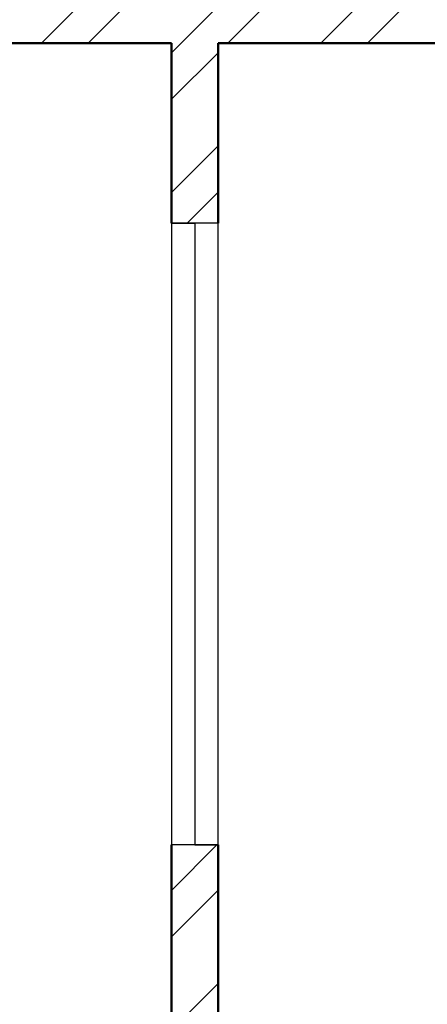
# Model space of a CAD drawing. Units: inches. Extents: x 963 to 2075, y 289 to 2657.
# Tile 61 of 98: x 1149 to 1188, y 2230 to 2325. Entities that reach past the tile are written whole.
import ezdxf

# ---------------------------------------------------------------- set-up
doc = ezdxf.new("R2010")
doc.units = ezdxf.units.IN
for name, color, linetype, lineweight in [('A-GLAZ', 3, 'Continuous', 25), ('A-WALL', 7, 'Continuous', 50), ('A-WALL-PATT', 8, 'Continuous', 13)]:
    doc.layers.add(name, color=color, linetype=linetype, lineweight=lineweight)

msp = doc.modelspace()

# ---------------------------------------------------------------- hatches: boundary and pattern name
at = {"layer": 'A-WALL-PATT'}
h = msp.add_hatch(dxfattribs=at)
h.set_pattern_fill('ANSI32', color=256)
h.paths.add_polyline_path([(1296.922, 2558.318), (1203.922, 2558.318), (1203.922, 2493.818), (1191.533, 2493.818), (1191.533, 2489.318), (1211.063, 2489.318), (1211.063, 2492.02), (1211.063, 2493.818), (1208.422, 2493.818), (1208.422, 2553.818), (1292.422, 2553.818), (1292.422, 2538.863), (1296.922, 2538.863)])
h.paths.add_polyline_path([(1442.422, 2558.318), (1349.422, 2558.318), (1349.422, 2538.943), (1353.922, 2538.943), (1353.922, 2553.818), (1437.922, 2553.818), (1437.922, 2493.818), (1434.542, 2493.818), (1434.542, 2489.318), (1448.311, 2489.318), (1448.311, 2491.568), (1448.311, 2493.818), (1442.422, 2493.818)])
h.paths.add_polyline_path([(1415.554, 2491.568), (1415.554, 2493.818), (1340.941, 2493.818), (1340.941, 2489.318), (1371.922, 2489.318), (1371.922, 2378.318), (1367.596, 2378.318), (1367.596, 2373.818), (1371.922, 2373.818), (1371.922, 2355.185), (1376.422, 2355.185), (1376.422, 2489.318), (1415.554, 2489.318)])
h.paths.add_polyline_path([(1304.941, 2491.568), (1304.941, 2493.818), (1296.922, 2493.818), (1296.922, 2514.863), (1292.422, 2514.863), (1292.422, 2493.818), (1232.808, 2493.818), (1232.808, 2489.318), (1256.422, 2489.318), (1256.422, 2327.318), (1253.714, 2327.318), (1253.714, 2322.818), (1328.422, 2322.818), (1328.422, 2331.147), (1323.922, 2331.147), (1323.922, 2327.318), (1260.922, 2327.318), (1260.922, 2373.818), (1323.922, 2373.818), (1323.922, 2357.812), (1328.422, 2357.812), (1328.422, 2373.818), (1346.007, 2373.818), (1346.007, 2376.068), (1346.007, 2378.318), (1260.922, 2378.318), (1260.922, 2489.318), (1304.941, 2489.318)])
h.paths.add_polyline_path([(1226.654, 2327.318), (1124.422, 2327.318), (1124.422, 2347.447), (1119.922, 2347.447), (1119.922, 2322.818), (1163.422, 2322.818), (1163.422, 2305.435), (1165.672, 2305.435), (1167.922, 2305.435), (1167.922, 2322.818), (1226.654, 2322.818), (1226.654, 2325.068)])
h.paths.add_polyline_path([(1095.922, 2489.318), (1124.422, 2489.318), (1131.533, 2489.318), (1131.533, 2491.568), (1131.533, 2493.818), (1119.922, 2493.818), (1091.422, 2493.818), (1091.422, 2417.318), (1095.922, 2417.318), (1119.922, 2417.318), (1119.922, 2407.447), (1124.422, 2407.447), (1124.422, 2421.818), (1095.922, 2421.818)])
h.paths.add_polyline_path([(1512.922, 2558.318), (1508.422, 2558.318), (1508.422, 2493.818), (1503.401, 2493.818), (1503.401, 2489.318), (1508.422, 2489.318), (1508.422, 2327.318), (1376.422, 2327.318), (1376.422, 2330.273), (1371.922, 2330.273), (1371.922, 2298.744), (1376.422, 2298.744), (1376.422, 2322.818), (1508.422, 2322.818), (1508.422, 2165.318), (1504.255, 2165.318), (1504.255, 2160.818), (1508.422, 2160.818), (1508.422, 2108.318), (1512.922, 2108.318), (1512.922, 2160.818), (1516.182, 2160.818), (1516.182, 2163.068), (1516.182, 2165.318), (1512.922, 2165.318), (1512.922, 2322.818), (1644.922, 2322.818), (1644.922, 2298.744), (1649.422, 2298.744), (1649.422, 2322.818), (1649.422, 2330.944), (1647.172, 2330.944), (1644.922, 2330.944), (1644.922, 2327.318), (1512.922, 2327.318), (1512.922, 2489.318), (1516.759, 2489.318), (1516.759, 2491.568), (1516.759, 2493.818), (1512.922, 2493.818)])
h.paths.add_polyline_path([(1671.922, 2558.318), (1578.922, 2558.318), (1578.922, 2493.818), (1573.526, 2493.818), (1573.526, 2489.318), (1586.537, 2489.318), (1586.537, 2491.568), (1586.537, 2493.818), (1583.422, 2493.818), (1583.422, 2553.818), (1667.422, 2553.818), (1667.422, 2541.109), (1671.922, 2541.109)])
h.paths.add_polyline_path([(1681.257, 2493.818), (1671.922, 2493.818), (1671.922, 2517.109), (1667.422, 2517.109), (1667.422, 2493.818), (1610.218, 2493.818), (1610.218, 2489.318), (1644.922, 2489.318), (1644.922, 2357.865), (1649.422, 2357.865), (1649.422, 2373.818), (1652.203, 2373.818), (1652.203, 2375.827), (1652.203, 2378.318), (1649.422, 2378.318), (1649.422, 2489.318), (1681.257, 2489.318), (1681.257, 2491.568)])
h.paths.add_polyline_path([(1821.922, 2558.318), (1728.922, 2558.318), (1728.922, 2541), (1733.422, 2541), (1733.422, 2553.818), (1817.422, 2553.818), (1817.422, 2493.818), (1813.507, 2493.818), (1813.507, 2489.318), (1830.078, 2489.318), (1830.078, 2491.568), (1830.078, 2493.818), (1821.922, 2493.818)])
h.paths.add_polyline_path([(1794.244, 2493.818), (1717.257, 2493.818), (1717.257, 2489.318), (1760.422, 2489.318), (1760.422, 2378.318), (1674.401, 2378.318), (1674.401, 2373.818), (1692.922, 2373.818), (1692.922, 2356.954), (1697.422, 2356.954), (1697.422, 2373.818), (1760.422, 2373.818), (1760.422, 2327.318), (1697.422, 2327.318), (1697.422, 2333.341), (1692.922, 2333.341), (1692.922, 2322.818), (1768.037, 2322.818), (1768.037, 2325.068), (1768.037, 2327.318), (1764.922, 2327.318), (1764.922, 2489.318), (1794.244, 2489.318)])
h.paths.add_polyline_path([(1733.422, 2517), (1728.922, 2517), (1728.922, 2493.818), (1733.422, 2493.818)], flags=17)
h.paths.add_polyline_path([(1929.922, 2493.818), (1890.078, 2493.818), (1890.078, 2489.318), (1896.922, 2489.318), (1925.422, 2489.318), (1925.422, 2421.818), (1896.922, 2421.818), (1896.922, 2408.318), (1901.422, 2408.318), (1901.422, 2417.318), (1925.422, 2417.318), (1929.922, 2417.318)])
h.paths.add_polyline_path([(1901.422, 2348.318), (1896.922, 2348.318), (1896.922, 2327.318), (1800.423, 2327.318), (1800.423, 2322.818), (1853.422, 2322.818), (1853.422, 2309.453), (1857.922, 2309.453), (1857.922, 2322.818), (1901.422, 2322.818)])
h.paths.add_polyline_path([(1857.922, 2249.453), (1853.422, 2249.453), (1853.422, 2214.818), (1686.309, 2214.818), (1686.309, 2210.318), (1853.422, 2210.318), (1853.422, 2202.134), (1857.922, 2202.134), (1857.922, 2210.318)])
h.paths.add_polyline_path([(1857.922, 2142.134), (1853.422, 2142.134), (1853.422, 2115.422), (1841.422, 2115.422), (1841.422, 2088.531), (1841.422, 2046.949), (1845.922, 2046.949), (1845.922, 2110.922), (1905.922, 2110.922), (1905.922, 2092.517), (1910.422, 2092.517), (1910.422, 2115.422), (1857.922, 2115.422)])
h.paths.add_polyline_path([(1532.436, 1482.342), (1573.456, 1482.342), (1573.456, 1501), (1532.436, 1501)], flags=9)
h.paths.add_polyline_path([(1438.658, 1486.302), (1479.678, 1486.302), (1479.678, 1504.96), (1438.658, 1504.96)], flags=9)
h.paths.add_polyline_path([(1411.215, 1365.308), (1659.139, 1365.308), (1659.139, 1402.401), (1411.215, 1402.401)], flags=9)
h.paths.add_polyline_path([(1185.671, 2296.298), (1248.16, 2296.298), (1248.16, 2314.955), (1185.671, 2314.955)], flags=9)
h.paths.add_polyline_path([(1177.31, 2187.35), (1216.15, 2187.35), (1216.15, 2206.007), (1177.31, 2206.007)], flags=9)
h.paths.add_polyline_path([(1295.101, 1602.083), (1328.26, 1602.083), (1328.26, 1620.741), (1295.101, 1620.741)], flags=9)
h.paths.add_polyline_path([(1525.126, 2005.99), (1558.39, 2005.99), (1558.39, 2024.648), (1525.126, 2024.648)], flags=9)
h.paths.add_polyline_path([(1459.606, 1977.125), (1472.195, 1977.125), (1472.195, 1987.429), (1459.606, 1987.429)], flags=9)
h.paths.add_polyline_path([(1467.815, 2053.676), (1480.018, 2053.676), (1480.018, 2063.979), (1467.815, 2063.979)], flags=9)
h.paths.add_polyline_path([(1555.184, 2119.02), (1584.563, 2119.02), (1584.563, 2137.678), (1555.184, 2137.678)], flags=25)
h.paths.add_polyline_path([(1405.389, 2115.291), (1444.478, 2115.291), (1444.478, 2133.948), (1405.389, 2133.948)], flags=25)
h.paths.add_polyline_path([(1698.482, 2004.259), (1727.695, 2004.259), (1727.695, 2022.916), (1698.482, 2022.916)], flags=9)
h.paths.add_polyline_path([(1612.158, 1972.855), (1629.016, 1972.855), (1629.016, 1983.159), (1612.158, 1983.159)], flags=9)
h.paths.add_polyline_path([(1608.289, 2060.036), (1625.147, 2060.036), (1625.147, 2070.34), (1608.289, 2070.34)], flags=9)
h.paths.add_polyline_path([(1527.954, 1684.402), (1566.795, 1684.402), (1566.795, 1703.06), (1527.954, 1703.06)], flags=9)
h.paths.add_polyline_path([(1422.792, 1683.59), (1461.633, 1683.59), (1461.633, 1702.247), (1422.792, 1702.247)], flags=9)
h.paths.add_polyline_path([(1531.262, 1732.459), (1574.015, 1732.459), (1574.015, 1751.116), (1531.262, 1751.116)], flags=9)
h.paths.add_polyline_path([(1402.872, 1732.845), (1439.799, 1732.845), (1439.799, 1751.502), (1402.872, 1751.502)], flags=9)
h.paths.add_polyline_path([(1243.122, 1923.132), (1281.962, 1923.132), (1281.962, 1941.79), (1243.122, 1941.79)], flags=9)
h.paths.add_polyline_path([(1181.752, 1792.268), (1244.241, 1792.268), (1244.241, 1810.926), (1181.752, 1810.926)], flags=9)
h.paths.add_polyline_path([(1265.822, 1670.3), (1316.071, 1670.3), (1316.071, 1688.957), (1265.822, 1688.957)], flags=9)
h.paths.add_polyline_path([(1140.263, 1676.054), (1179.104, 1676.054), (1179.104, 1694.711), (1140.263, 1694.711)], flags=9)
h.paths.add_polyline_path([(1107.49, 1490.889), (1143.374, 1490.889), (1143.374, 1509.546), (1107.49, 1509.546)], flags=9)
h.paths.add_polyline_path([(1217.584, 1483.899), (1246.741, 1483.899), (1246.741, 1502.556), (1217.584, 1502.556)], flags=9)
h.paths.add_polyline_path([(1389.21, 1486.919), (1418.367, 1486.919), (1418.367, 1505.576), (1389.21, 1505.576)], flags=9)
h.paths.add_polyline_path([(1672.208, 1602.083), (1705.366, 1602.083), (1705.366, 1620.741), (1672.208, 1620.741)], flags=9)
h.paths.add_polyline_path([(1752.082, 1522.638), (1781.24, 1522.638), (1781.24, 1541.295), (1752.082, 1541.295)], flags=9)
h.paths.add_polyline_path([(1848.275, 1491.26), (1884.158, 1491.26), (1884.158, 1509.918), (1848.275, 1509.918)], flags=9)
h.paths.add_polyline_path([(1822.47, 1685.62), (1861.31, 1685.62), (1861.31, 1704.278), (1822.47, 1704.278)], flags=9)
h.paths.add_polyline_path([(1713.195, 1672.232), (1763.444, 1672.232), (1763.444, 1690.889), (1713.195, 1690.889)], flags=9)
h.paths.add_polyline_path([(1736.619, 1790.578), (1799.109, 1790.578), (1799.109, 1809.235), (1736.619, 1809.235)], flags=9)
h.paths.add_polyline_path([(1691.491, 1916.355), (1730.332, 1916.355), (1730.332, 1935.013), (1691.491, 1935.013)], flags=9)
h.paths.add_polyline_path([(1764.872, 1973.922), (1794.306, 1973.922), (1794.306, 1992.58), (1764.872, 1992.58)], flags=9)
h.paths.add_polyline_path([(1767.854, 2034.017), (1797.288, 2034.017), (1797.288, 2052.674), (1767.854, 2052.674)], flags=9)
h.paths.add_polyline_path([(1851.593, 2060.331), (1880.751, 2060.331), (1880.751, 2078.989), (1851.593, 2078.989)], flags=25)
h.paths.add_polyline_path([(1688.491, 2086.874), (1727.332, 2086.874), (1727.332, 2105.531), (1688.491, 2105.531)], flags=9)
h.paths.add_polyline_path([(1537.743, 2293.581), (1580.495, 2293.581), (1580.495, 2312.239), (1537.743, 2312.239)], flags=25)
h.paths.add_polyline_path([(1425.587, 2296.109), (1468.34, 2296.109), (1468.34, 2314.766), (1425.587, 2314.766)], flags=25)
h.paths.add_polyline_path([(1278.518, 2004.184), (1307.72, 2004.184), (1307.72, 2022.841), (1278.518, 2022.841)], flags=9)
h.paths.add_polyline_path([(1193.282, 1973.635), (1222.715, 1973.635), (1222.715, 1992.292), (1193.282, 1992.292)], flags=9)
h.paths.add_polyline_path([(1192.411, 2040.577), (1221.845, 2040.577), (1221.845, 2059.234), (1192.411, 2059.234)], flags=9)
h.paths.add_polyline_path([(1130.603, 1951.393), (1159.76, 1951.393), (1159.76, 1970.05), (1130.603, 1970.05)], flags=9)
h.paths.add_polyline_path([(1132.827, 2052.494), (1161.984, 2052.494), (1161.984, 2071.151), (1132.827, 2071.151)], flags=9)
h.paths.add_polyline_path([(1265.128, 2334.619), (1315.377, 2334.619), (1315.377, 2353.277), (1265.128, 2353.277)], flags=25)
h.paths.add_polyline_path([(1136.741, 2330.785), (1175.582, 2330.785), (1175.582, 2349.443), (1136.741, 2349.443)], flags=9)
h.paths.add_polyline_path([(1287.422, 2417.204), (1320.58, 2417.204), (1320.58, 2435.861), (1287.422, 2435.861)], flags=25)
h.paths.add_polyline_path([(1430.988, 2329.159), (1469.828, 2329.159), (1469.828, 2347.816), (1430.988, 2347.816)], flags=25)
h.paths.add_polyline_path([(1525.424, 2329.213), (1564.264, 2329.213), (1564.264, 2347.87), (1525.424, 2347.87)], flags=25)
h.paths.add_polyline_path([(1684.525, 2382.799), (1717.683, 2382.799), (1717.683, 2401.457), (1684.525, 2401.457)], flags=25)
h.paths.add_polyline_path([(1704.805, 2340.293), (1755.054, 2340.293), (1755.054, 2358.95), (1704.805, 2358.95)], flags=25)
h.paths.add_polyline_path([(1694.113, 2287.757), (1756.602, 2287.757), (1756.602, 2306.414), (1694.113, 2306.414)], flags=9)
h.paths.add_polyline_path([(1815.778, 2329.861), (1854.618, 2329.861), (1854.618, 2348.518), (1815.778, 2348.518)], flags=9)
h.paths.add_polyline_path([(1842.873, 2514.256), (1878.756, 2514.256), (1878.756, 2532.914), (1842.873, 2532.914)], flags=9)
h.paths.add_polyline_path([(1769.513, 2531.447), (1798.671, 2531.447), (1798.671, 2550.104), (1769.513, 2550.104)], flags=25)
h.paths.add_polyline_path([(1594.772, 2518.468), (1623.93, 2518.468), (1623.93, 2537.125), (1594.772, 2537.125)], flags=25)
h.paths.add_polyline_path([(1520.723, 2516.185), (1556.606, 2516.185), (1556.606, 2534.842), (1520.723, 2534.842)], flags=25)
h.paths.add_polyline_path([(1464.456, 2516.694), (1500.34, 2516.694), (1500.34, 2535.351), (1464.456, 2535.351)], flags=25)
h.paths.add_polyline_path([(1365.696, 2528.97), (1394.854, 2528.97), (1394.854, 2547.627), (1365.696, 2547.627)], flags=25)
h.paths.add_polyline_path([(1222.838, 2516.231), (1251.995, 2516.231), (1251.995, 2534.889), (1222.838, 2534.889)], flags=25)
h.paths.add_polyline_path([(1104.545, 2509.6), (1140.429, 2509.6), (1140.429, 2528.257), (1104.545, 2528.257)], flags=9)
h = msp.add_hatch(dxfattribs=at)
h.set_pattern_fill('ANSI32', color=256)
h.paths.add_polyline_path([(1335.968, 2212.568), (1335.968, 2214.818), (1167.922, 2214.818), (1167.922, 2245.435), (1163.422, 2245.435), (1163.422, 2210.318), (1163.422, 2194.812), (1167.922, 2194.812), (1167.922, 2210.318), (1335.968, 2210.318)])
h.paths.add_polyline_path([(1532.436, 1482.342), (1573.456, 1482.342), (1573.456, 1501), (1532.436, 1501)], flags=9)
h.paths.add_polyline_path([(1438.658, 1486.302), (1479.678, 1486.302), (1479.678, 1504.96), (1438.658, 1504.96)], flags=9)
h.paths.add_polyline_path([(1411.215, 1365.308), (1659.139, 1365.308), (1659.139, 1402.401), (1411.215, 1402.401)], flags=9)
h.paths.add_polyline_path([(1185.671, 2296.298), (1248.16, 2296.298), (1248.16, 2314.955), (1185.671, 2314.955)], flags=9)
h.paths.add_polyline_path([(1177.31, 2187.35), (1216.15, 2187.35), (1216.15, 2206.007), (1177.31, 2206.007)], flags=9)
h.paths.add_polyline_path([(1295.101, 1602.083), (1328.26, 1602.083), (1328.26, 1620.741), (1295.101, 1620.741)], flags=9)
h.paths.add_polyline_path([(1525.126, 2005.99), (1558.39, 2005.99), (1558.39, 2024.648), (1525.126, 2024.648)], flags=9)
h.paths.add_polyline_path([(1459.606, 1977.125), (1472.195, 1977.125), (1472.195, 1987.429), (1459.606, 1987.429)], flags=9)
h.paths.add_polyline_path([(1467.815, 2053.676), (1480.018, 2053.676), (1480.018, 2063.979), (1467.815, 2063.979)], flags=9)
h.paths.add_polyline_path([(1555.184, 2119.02), (1584.563, 2119.02), (1584.563, 2137.678), (1555.184, 2137.678)], flags=9)
h.paths.add_polyline_path([(1405.389, 2115.291), (1444.478, 2115.291), (1444.478, 2133.948), (1405.389, 2133.948)], flags=9)
h.paths.add_polyline_path([(1698.482, 2004.259), (1727.695, 2004.259), (1727.695, 2022.916), (1698.482, 2022.916)], flags=9)
h.paths.add_polyline_path([(1612.158, 1972.855), (1629.016, 1972.855), (1629.016, 1983.159), (1612.158, 1983.159)], flags=9)
h.paths.add_polyline_path([(1608.289, 2060.036), (1625.147, 2060.036), (1625.147, 2070.34), (1608.289, 2070.34)], flags=9)
h.paths.add_polyline_path([(1527.954, 1684.402), (1566.795, 1684.402), (1566.795, 1703.06), (1527.954, 1703.06)], flags=9)
h.paths.add_polyline_path([(1422.792, 1683.59), (1461.633, 1683.59), (1461.633, 1702.247), (1422.792, 1702.247)], flags=9)
h.paths.add_polyline_path([(1531.262, 1732.459), (1574.015, 1732.459), (1574.015, 1751.116), (1531.262, 1751.116)], flags=9)
h.paths.add_polyline_path([(1402.872, 1732.845), (1439.799, 1732.845), (1439.799, 1751.502), (1402.872, 1751.502)], flags=9)
h.paths.add_polyline_path([(1243.122, 1923.132), (1281.962, 1923.132), (1281.962, 1941.79), (1243.122, 1941.79)], flags=9)
h.paths.add_polyline_path([(1181.752, 1792.268), (1244.241, 1792.268), (1244.241, 1810.926), (1181.752, 1810.926)], flags=9)
h.paths.add_polyline_path([(1265.822, 1670.3), (1316.071, 1670.3), (1316.071, 1688.957), (1265.822, 1688.957)], flags=9)
h.paths.add_polyline_path([(1140.263, 1676.054), (1179.104, 1676.054), (1179.104, 1694.711), (1140.263, 1694.711)], flags=9)
h.paths.add_polyline_path([(1107.49, 1490.889), (1143.374, 1490.889), (1143.374, 1509.546), (1107.49, 1509.546)], flags=9)
h.paths.add_polyline_path([(1217.584, 1483.899), (1246.741, 1483.899), (1246.741, 1502.556), (1217.584, 1502.556)], flags=9)
h.paths.add_polyline_path([(1389.21, 1486.919), (1418.367, 1486.919), (1418.367, 1505.576), (1389.21, 1505.576)], flags=9)
h.paths.add_polyline_path([(1672.208, 1602.083), (1705.366, 1602.083), (1705.366, 1620.741), (1672.208, 1620.741)], flags=9)
h.paths.add_polyline_path([(1752.082, 1522.638), (1781.24, 1522.638), (1781.24, 1541.295), (1752.082, 1541.295)], flags=9)
h.paths.add_polyline_path([(1848.275, 1491.26), (1884.158, 1491.26), (1884.158, 1509.918), (1848.275, 1509.918)], flags=9)
h.paths.add_polyline_path([(1822.47, 1685.62), (1861.31, 1685.62), (1861.31, 1704.278), (1822.47, 1704.278)], flags=9)
h.paths.add_polyline_path([(1713.195, 1672.232), (1763.444, 1672.232), (1763.444, 1690.889), (1713.195, 1690.889)], flags=9)
h.paths.add_polyline_path([(1736.619, 1790.578), (1799.109, 1790.578), (1799.109, 1809.235), (1736.619, 1809.235)], flags=9)
h.paths.add_polyline_path([(1691.491, 1916.355), (1730.332, 1916.355), (1730.332, 1935.013), (1691.491, 1935.013)], flags=9)
h.paths.add_polyline_path([(1764.872, 1973.922), (1794.306, 1973.922), (1794.306, 1992.58), (1764.872, 1992.58)], flags=9)
h.paths.add_polyline_path([(1767.854, 2034.017), (1797.288, 2034.017), (1797.288, 2052.674), (1767.854, 2052.674)], flags=9)
h.paths.add_polyline_path([(1851.593, 2060.331), (1880.751, 2060.331), (1880.751, 2078.989), (1851.593, 2078.989)], flags=9)
h.paths.add_polyline_path([(1688.491, 2086.874), (1727.332, 2086.874), (1727.332, 2105.531), (1688.491, 2105.531)], flags=9)
h.paths.add_polyline_path([(1537.743, 2293.581), (1580.495, 2293.581), (1580.495, 2312.239), (1537.743, 2312.239)], flags=9)
h.paths.add_polyline_path([(1425.587, 2296.109), (1468.34, 2296.109), (1468.34, 2314.766), (1425.587, 2314.766)], flags=9)
h.paths.add_polyline_path([(1278.518, 2004.184), (1307.72, 2004.184), (1307.72, 2022.841), (1278.518, 2022.841)], flags=9)
h.paths.add_polyline_path([(1193.282, 1973.635), (1222.715, 1973.635), (1222.715, 1992.292), (1193.282, 1992.292)], flags=9)
h.paths.add_polyline_path([(1192.411, 2040.577), (1221.845, 2040.577), (1221.845, 2059.234), (1192.411, 2059.234)], flags=9)
h.paths.add_polyline_path([(1130.603, 1951.393), (1159.76, 1951.393), (1159.76, 1970.05), (1130.603, 1970.05)], flags=9)
h.paths.add_polyline_path([(1132.827, 2052.494), (1161.984, 2052.494), (1161.984, 2071.151), (1132.827, 2071.151)], flags=9)
h.paths.add_polyline_path([(1265.128, 2334.619), (1315.377, 2334.619), (1315.377, 2353.277), (1265.128, 2353.277)], flags=9)
h.paths.add_polyline_path([(1136.741, 2330.785), (1175.582, 2330.785), (1175.582, 2349.443), (1136.741, 2349.443)], flags=9)
h.paths.add_polyline_path([(1287.422, 2417.204), (1320.58, 2417.204), (1320.58, 2435.861), (1287.422, 2435.861)], flags=9)
h.paths.add_polyline_path([(1430.988, 2329.159), (1469.828, 2329.159), (1469.828, 2347.816), (1430.988, 2347.816)], flags=9)
h.paths.add_polyline_path([(1525.424, 2329.213), (1564.264, 2329.213), (1564.264, 2347.87), (1525.424, 2347.87)], flags=9)
h.paths.add_polyline_path([(1684.525, 2382.799), (1717.683, 2382.799), (1717.683, 2401.457), (1684.525, 2401.457)], flags=9)
h.paths.add_polyline_path([(1704.805, 2340.293), (1755.054, 2340.293), (1755.054, 2358.95), (1704.805, 2358.95)], flags=9)
h.paths.add_polyline_path([(1694.113, 2287.757), (1756.602, 2287.757), (1756.602, 2306.414), (1694.113, 2306.414)], flags=9)
h.paths.add_polyline_path([(1815.778, 2329.861), (1854.618, 2329.861), (1854.618, 2348.518), (1815.778, 2348.518)], flags=9)
h.paths.add_polyline_path([(1842.873, 2514.256), (1878.756, 2514.256), (1878.756, 2532.914), (1842.873, 2532.914)], flags=9)
h.paths.add_polyline_path([(1769.513, 2531.447), (1798.671, 2531.447), (1798.671, 2550.104), (1769.513, 2550.104)], flags=9)
h.paths.add_polyline_path([(1594.772, 2518.468), (1623.93, 2518.468), (1623.93, 2537.125), (1594.772, 2537.125)], flags=9)
h.paths.add_polyline_path([(1520.723, 2516.185), (1556.606, 2516.185), (1556.606, 2534.842), (1520.723, 2534.842)], flags=9)
h.paths.add_polyline_path([(1464.456, 2516.694), (1500.34, 2516.694), (1500.34, 2535.351), (1464.456, 2535.351)], flags=9)
h.paths.add_polyline_path([(1365.696, 2528.97), (1394.854, 2528.97), (1394.854, 2547.627), (1365.696, 2547.627)], flags=9)
h.paths.add_polyline_path([(1222.838, 2516.231), (1251.995, 2516.231), (1251.995, 2534.889), (1222.838, 2534.889)], flags=9)
h.paths.add_polyline_path([(1104.545, 2509.6), (1140.429, 2509.6), (1140.429, 2528.257), (1104.545, 2528.257)], flags=9)

# ---------------------------------------------------------------- linework, layer by layer
at = {"layer": 'A-GLAZ'}
for p, q in [((1167.922, 2305.435), (1163.422, 2305.435)), ((1163.422, 2305.435), (1165.672, 2305.435)), ((1163.422, 2305.435), (1163.422, 2245.435)), ((1165.672, 2305.435), (1165.672, 2245.435)), ((1167.922, 2245.435), (1167.922, 2305.435)), ((1167.922, 2245.435), (1163.422, 2245.435)), ((1165.672, 2245.435), (1167.922, 2245.435))]:
    msp.add_line(p, q, dxfattribs=at)
at = {"layer": 'A-WALL'}
for p, q in [((1119.922, 2322.818), (1163.422, 2322.818)), ((1163.422, 2322.818), (1163.422, 2305.435)), ((1167.922, 2322.818), (1167.922, 2305.435)), ((1167.922, 2322.818), (1226.654, 2322.818)), ((1163.422, 2245.435), (1163.422, 2210.318)), ((1167.922, 2245.435), (1167.922, 2214.818))]:
    msp.add_line(p, q, dxfattribs=at)

doc.saveas('drawing.dxf')
